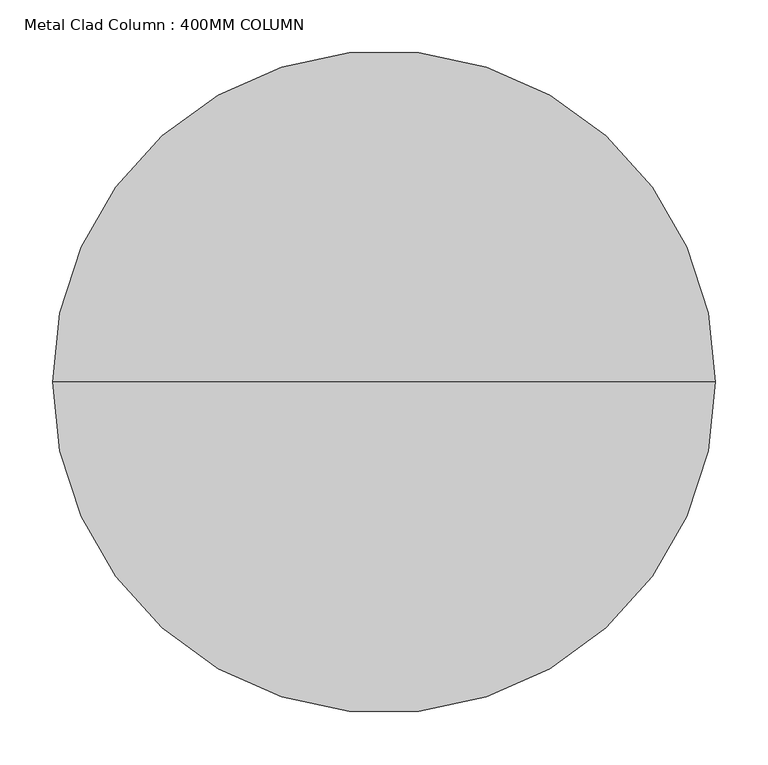
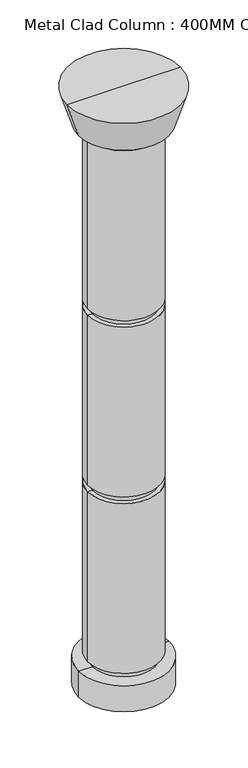
"""IFC4 building model written with IfcOpenShell, lengths in millimetres: column geometry, Metal Clad Column : 400MM COLUMN."""

from ifc_helpers import new_model, si_unit, frame, origin, place, context, project, spatial, polyline, circle_curve, source, transform, mapped, element, save
from ifc_brep_helpers import plane_surface, cylinder_surface, revolved_surface, advanced_brep


def metal_clad_column_400mm_column_d615f8bc(model_context):
    return source(origin(), model_context, "Body", "AdvancedBrep", [
        advanced_brep(
        [(0.0, 0.0, -100.0), (250.8, 0.0, -100.0), (-250.8, 0.0, -100.0), (250.8, 0.0, 52.4), (-250.8, 0.0, 52.4), (174.6, 0.0, 1125.9333333), (200.0, 0.0, 1125.9333333), (-200.0, 0.0, 1125.9333333), (-174.6, 0.0, 1125.9333333), (200.0, 0.0, 2123.2666667), (-200.0, 0.0, 2123.2666667), (174.6, 0.0, 1087.8333333), (-174.6, 0.0, 1087.8333333), (200.0, 0.0, 1087.8333333), (-200.0, 0.0, 1087.8333333), (200.0, 0.0, 90.5), (-200.0, 0.0, 90.5), (174.6, 0.0, 90.5), (-174.6, 0.0, 90.5), (174.6, 0.0, 52.4), (-174.6, 0.0, 52.4), (250.8, 0.0, 3196.8), (314.3, 0.0, 3400.0), (-314.3, 0.0, 3400.0), (-250.8, 0.0, 3196.8), (0.0, 0.0, 3400.0), (174.6, 0.0, 3196.8), (-174.6, 0.0, 3196.8), (174.6, 0.0, 3158.7), (-174.6, 0.0, 3158.7), (200.0, 0.0, 3158.7), (-200.0, 0.0, 3158.7), (200.0, 0.0, 2161.3666667), (-200.0, 0.0, 2161.3666667), (174.6, 0.0, 2161.3666667), (-174.6, 0.0, 2161.3666667), (174.6, 0.0, 2123.2666667), (-174.6, 0.0, 2123.2666667)],
        [
            (0, 1),
            (1, 2, circle_curve(frame((0.0, 0.0, -100.0), z_axis=(0.0, 0.0, -1.0), x_axis=(-1.0, 0.0, 0.0)), 250.8)),
            (2, 0),
            (2, 1, circle_curve(frame((0.0, 0.0, -100.0), z_axis=(0.0, 0.0, -1.0), x_axis=(-1.0, 0.0, 0.0)), 250.8)),
            (1, 3),
            (3, 4, circle_curve(frame((0.0, 0.0, 52.4), z_axis=(0.0, 0.0, -1.0), x_axis=(-1.0, 0.0, 0.0)), 250.8)),
            (4, 2),
            (4, 3, circle_curve(frame((0.0, 0.0, 52.4), z_axis=(0.0, 0.0, -1.0), x_axis=(-1.0, 0.0, 0.0)), 250.8)),
            (5, 6),
            (6, 7, circle_curve(frame((0.0, 0.0, 1125.9333333), z_axis=(0.0, 0.0, -1.0), x_axis=(-1.0, 0.0, 0.0)), 200.0)),
            (7, 8),
            (8, 5, circle_curve(frame((0.0, 0.0, 1125.9333333), z_axis=(0.0, 0.0, 1.0), x_axis=(-1.0, 0.0, 0.0)), 174.6)),
            (6, 9),
            (9, 10, circle_curve(frame((0.0, 0.0, 2123.2666667), z_axis=(0.0, 0.0, -1.0), x_axis=(-1.0, 0.0, 0.0)), 200.0)),
            (10, 7),
            (10, 9, circle_curve(frame((0.0, 0.0, 2123.2666667), z_axis=(0.0, 0.0, -1.0), x_axis=(-1.0, 0.0, 0.0)), 200.0)),
            (6, 7, circle_curve(frame((0.0, 0.0, 1125.9333333), z_axis=(0.0, 0.0, 1.0), x_axis=(-1.0, 0.0, 0.0)), 200.0)),
            (5, 8, circle_curve(frame((0.0, 0.0, 1125.9333333), z_axis=(0.0, 0.0, 1.0), x_axis=(-1.0, 0.0, 0.0)), 174.6)),
            (11, 5),
            (8, 12),
            (12, 11, circle_curve(frame((0.0, 0.0, 1087.8333333), z_axis=(0.0, 0.0, 1.0), x_axis=(-1.0, 0.0, 0.0)), 174.6)),
            (11, 12, circle_curve(frame((0.0, 0.0, 1087.8333333), z_axis=(0.0, 0.0, 1.0), x_axis=(-1.0, 0.0, 0.0)), 174.6)),
            (13, 11),
            (12, 14),
            (14, 13, circle_curve(frame((0.0, 0.0, 1087.8333333), z_axis=(0.0, 0.0, 1.0), x_axis=(-1.0, 0.0, 0.0)), 200.0)),
            (13, 14, circle_curve(frame((0.0, 0.0, 1087.8333333), z_axis=(0.0, 0.0, 1.0), x_axis=(-1.0, 0.0, 0.0)), 200.0)),
            (15, 13),
            (14, 16),
            (16, 15, circle_curve(frame((0.0, 0.0, 90.5), z_axis=(0.0, 0.0, 1.0), x_axis=(-1.0, 0.0, 0.0)), 200.0)),
            (15, 16, circle_curve(frame((0.0, 0.0, 90.5), z_axis=(0.0, 0.0, 1.0), x_axis=(-1.0, 0.0, 0.0)), 200.0)),
            (17, 15),
            (16, 18),
            (18, 17, circle_curve(frame((0.0, 0.0, 90.5), z_axis=(0.0, 0.0, 1.0), x_axis=(-1.0, 0.0, 0.0)), 174.6)),
            (17, 18, circle_curve(frame((0.0, 0.0, 90.5), z_axis=(0.0, 0.0, 1.0), x_axis=(-1.0, 0.0, 0.0)), 174.6)),
            (19, 17),
            (18, 20),
            (20, 19, circle_curve(frame((0.0, 0.0, 52.4), z_axis=(0.0, 0.0, 1.0), x_axis=(-1.0, 0.0, 0.0)), 174.6)),
            (19, 20, circle_curve(frame((0.0, 0.0, 52.4), z_axis=(0.0, 0.0, 1.0), x_axis=(-1.0, 0.0, 0.0)), 174.6)),
            (3, 19),
            (20, 4),
            (21, 22),
            (22, 23, circle_curve(frame((0.0, 0.0, 3400.0), z_axis=(0.0, 0.0, -1.0), x_axis=(-1.0, 0.0, 0.0)), 314.3)),
            (23, 24),
            (24, 21, circle_curve(frame((0.0, 0.0, 3196.8), z_axis=(0.0, 0.0, 1.0), x_axis=(-1.0, 0.0, 0.0)), 250.8)),
            (22, 25),
            (25, 23),
            (22, 23, circle_curve(frame((0.0, 0.0, 3400.0), z_axis=(0.0, 0.0, 1.0), x_axis=(-1.0, 0.0, 0.0)), 314.3)),
            (21, 24, circle_curve(frame((0.0, 0.0, 3196.8), z_axis=(0.0, 0.0, 1.0), x_axis=(-1.0, 0.0, 0.0)), 250.8)),
            (26, 21),
            (24, 27),
            (27, 26, circle_curve(frame((0.0, 0.0, 3196.8), z_axis=(0.0, 0.0, 1.0), x_axis=(-1.0, 0.0, 0.0)), 174.6)),
            (26, 27, circle_curve(frame((0.0, 0.0, 3196.8), z_axis=(0.0, 0.0, 1.0), x_axis=(-1.0, 0.0, 0.0)), 174.6)),
            (28, 26),
            (27, 29),
            (29, 28, circle_curve(frame((0.0, 0.0, 3158.7), z_axis=(0.0, 0.0, 1.0), x_axis=(-1.0, 0.0, 0.0)), 174.6)),
            (28, 29, circle_curve(frame((0.0, 0.0, 3158.7), z_axis=(0.0, 0.0, 1.0), x_axis=(-1.0, 0.0, 0.0)), 174.6)),
            (30, 28),
            (29, 31),
            (31, 30, circle_curve(frame((0.0, 0.0, 3158.7), z_axis=(0.0, 0.0, 1.0), x_axis=(-1.0, 0.0, 0.0)), 200.0)),
            (30, 31, circle_curve(frame((0.0, 0.0, 3158.7), z_axis=(0.0, 0.0, 1.0), x_axis=(-1.0, 0.0, 0.0)), 200.0)),
            (32, 30),
            (31, 33),
            (33, 32, circle_curve(frame((0.0, 0.0, 2161.3666667), z_axis=(0.0, 0.0, 1.0), x_axis=(-1.0, 0.0, 0.0)), 200.0)),
            (32, 33, circle_curve(frame((0.0, 0.0, 2161.3666667), z_axis=(0.0, 0.0, 1.0), x_axis=(-1.0, 0.0, 0.0)), 200.0)),
            (34, 32),
            (33, 35),
            (35, 34, circle_curve(frame((0.0, 0.0, 2161.3666667), z_axis=(0.0, 0.0, 1.0), x_axis=(-1.0, 0.0, 0.0)), 174.6)),
            (34, 35, circle_curve(frame((0.0, 0.0, 2161.3666667), z_axis=(0.0, 0.0, 1.0), x_axis=(-1.0, 0.0, 0.0)), 174.6)),
            (36, 34),
            (35, 37),
            (37, 36, circle_curve(frame((0.0, 0.0, 2123.2666667), z_axis=(0.0, 0.0, 1.0), x_axis=(-1.0, 0.0, 0.0)), 174.6)),
            (36, 37, circle_curve(frame((0.0, 0.0, 2123.2666667), z_axis=(0.0, 0.0, 1.0), x_axis=(-1.0, 0.0, 0.0)), 174.6)),
            (9, 36),
            (37, 10),
        ],
        [
            plane_surface(frame((0.0, 0.0, -100.0), z_axis=(0.0, 0.0, -1.0), x_axis=(-1.0, 0.0, 0.0))),
            cylinder_surface(frame((0.0, 0.0, 3400.0), z_axis=(0.0, 0.0, -1.0), x_axis=(-1.0, 0.0, 0.0)), 250.8),
            plane_surface(frame((0.0, 0.0, 1125.9333333), z_axis=(0.0, 0.0, -1.0), x_axis=(-1.0, 0.0, 0.0))),
            cylinder_surface(frame((0.0, 0.0, 3400.0), z_axis=(0.0, 0.0, -1.0), x_axis=(-1.0, 0.0, 0.0)), 200.0),
            cylinder_surface(frame((0.0, 0.0, 3400.0), z_axis=(0.0, 0.0, -1.0), x_axis=(-1.0, 0.0, 0.0)), 174.6),
            plane_surface(frame((0.0, 0.0, 1087.8333333), z_axis=(0.0, 0.0, 1.0), x_axis=(-1.0, 0.0, 0.0))),
            plane_surface(frame((0.0, 0.0, 90.5), z_axis=(0.0, 0.0, -1.0), x_axis=(-1.0, 0.0, 0.0))),
            plane_surface(frame((0.0, 0.0, 52.4), z_axis=(0.0, 0.0, 1.0), x_axis=(-1.0, 0.0, 0.0))),
            revolved_surface(polyline([(-314.3, 0.0, 3400.0), (-250.8, 0.0, 3196.8)]), (0.0, 0.0, 3400.0), (0.0, 0.0, -1.0)),
            plane_surface(frame((0.0, 0.0, 3400.0), z_axis=(0.0, 0.0, 1.0), x_axis=(-1.0, 0.0, 0.0))),
            plane_surface(frame((0.0, 0.0, 3196.8), z_axis=(0.0, 0.0, -1.0), x_axis=(-1.0, 0.0, 0.0))),
            plane_surface(frame((0.0, 0.0, 3158.7), z_axis=(0.0, 0.0, 1.0), x_axis=(-1.0, 0.0, 0.0))),
            plane_surface(frame((0.0, 0.0, 2161.3666667), z_axis=(0.0, 0.0, -1.0), x_axis=(-1.0, 0.0, 0.0))),
            plane_surface(frame((0.0, 0.0, 2123.2666667), z_axis=(0.0, 0.0, 1.0), x_axis=(-1.0, 0.0, 0.0))),
        ],
        [
            (0, [[1, 2, 3]]),
            (0, [[-3, 4, -1]]),
            (1, [[5, 6, 7, -2]]),
            (1, [[-7, 8, -5, -4]]),
            (2, [[9, 10, 11, 12]]),
            (3, [[13, 14, 15, -10]]),
            (3, [[-15, 16, -13, 17]]),
            (2, [[-11, -17, -9, 18]]),
            (4, [[19, -12, 20, 21]]),
            (4, [[-20, -18, -19, 22]]),
            (5, [[23, -21, 24, 25]]),
            (5, [[-24, -22, -23, 26]]),
            (3, [[27, -25, 28, 29]]),
            (3, [[-28, -26, -27, 30]]),
            (6, [[31, -29, 32, 33]]),
            (6, [[-32, -30, -31, 34]]),
            (4, [[35, -33, 36, 37]]),
            (4, [[-36, -34, -35, 38]]),
            (7, [[39, -37, 40, -6]]),
            (7, [[-40, -38, -39, -8]]),
            (8, [[41, 42, 43, 44]]),
            (9, [[45, 46, -42]]),
            (9, [[-46, -45, 47]]),
            (8, [[-43, -47, -41, 48]]),
            (10, [[49, -44, 50, 51]]),
            (10, [[-50, -48, -49, 52]]),
            (4, [[53, -51, 54, 55]]),
            (4, [[-54, -52, -53, 56]]),
            (11, [[57, -55, 58, 59]]),
            (11, [[-58, -56, -57, 60]]),
            (3, [[61, -59, 62, 63]]),
            (3, [[-62, -60, -61, 64]]),
            (12, [[65, -63, 66, 67]]),
            (12, [[-66, -64, -65, 68]]),
            (4, [[69, -67, 70, 71]]),
            (4, [[-70, -68, -69, 72]]),
            (13, [[73, -71, 74, -14]]),
            (13, [[-74, -72, -73, -16]]),
        ],
    ),
    ])


if __name__ == "__main__":
    model = new_model("IFC4")
    model_context = context("Model", 3, world=origin())
    ifc_project = project(units=[si_unit("LENGTHUNIT", "METRE", prefix="MILLI")], contexts=[model_context])
    site = spatial("IfcSite", under=ifc_project)
    building = spatial("IfcBuilding", under=site)
    placement = place(None, origin())
    metal_clad_column_400mm_column_shape = metal_clad_column_400mm_column_d615f8bc(model_context)
    element("IfcColumn", 1, ObjectType="Metal Clad Column : 400MM COLUMN", at=placement, inside=building, context=model_context, shape_type="MappedRepresentation", body=[
        mapped(metal_clad_column_400mm_column_shape, transform((0.0, 0.0, 0.0), x_axis=(1.0, 0.0, 0.0), y_axis=(0.0, 1.0, 0.0), z_axis=(0.0, 0.0, 1.0))),
    ])
    save(model, "model.ifc")

# Revit data of these elements
# Type "Metal Clad Column : 400MM COLUMN"
#   Assembly Code = "B1010200"
#   Base = 0' - 6"
#   Capital = 0' - 8"
#   Diameter = 1' - 3.74803"
#   Joint Depth = 0' - 1"
#   Joint Width = 0' - 1 1/2"
#   Offset base level = 0' - 0"
#   Offset top level = 0' - 0"
#   Material = Aluminum
# Element 1 (IfcColumn, "Metal Clad Column : 400MM COLUMN")
#   Materials on its faces: "Aluminum"
# Materials
#   "Aluminum": class "Metal", colour RGB 247 247 247, transparency 0, Description = "Aluminum 6061", Cost = 0
